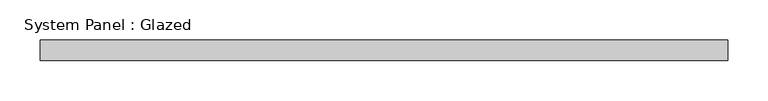
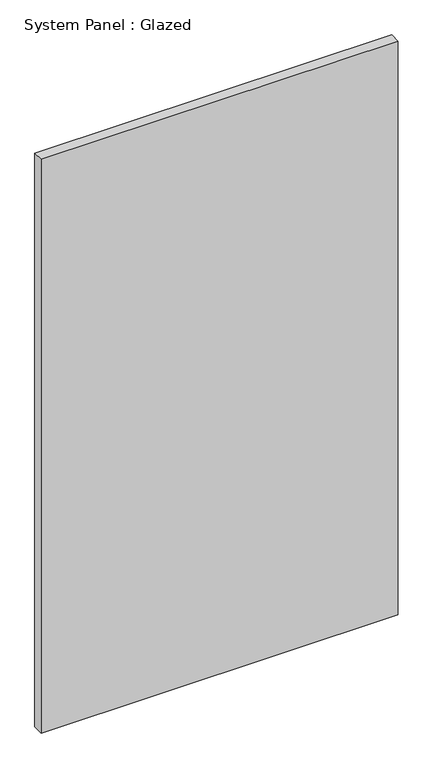
"""IFC4 building model written with IfcOpenShell, lengths in millimetres: plate geometry, System Panel : Glazed."""

from ifc_helpers import new_model, si_unit, origin, origin_with_axes, place, context, project, spatial, polyline, outline, extrude, source, transform, mapped, element, save


def system_panel_glazed_14014958(model_context):
    return source(origin(), model_context, "Body", "SweptSolid", [
        extrude(outline(polyline([(425.45, 19.05), (-425.45, 19.05), (-425.45, 44.45), (425.45, 44.45), (425.45, 19.05)])), origin_with_axes(), (0.0, 0.0, 1.0), 1444.0246189),
    ])


if __name__ == "__main__":
    model = new_model("IFC4")
    model_context = context("Model", 3, world=origin())
    ifc_project = project(units=[si_unit("LENGTHUNIT", "METRE", prefix="MILLI")], contexts=[model_context])
    site = spatial("IfcSite", under=ifc_project)
    building = spatial("IfcBuilding", under=site)
    placement = place(None, origin())
    system_panel_glazed_shape = system_panel_glazed_14014958(model_context)
    element("IfcPlate", 1, ObjectType="System Panel : Glazed", at=placement, inside=building, context=model_context, shape_type="MappedRepresentation", body=[
        mapped(system_panel_glazed_shape, transform((0.0, 0.0, 0.0), x_axis=(1.0, 0.0, 0.0), y_axis=(0.0, 1.0, 0.0), z_axis=(0.0, 0.0, 1.0))),
    ])
    save(model, "model.ifc")

# Revit data of these elements
# Type "System Panel : Glazed"
#   Construction Type Id = "GSP4R"
#   Analytic Construction = "1/8 in Pilkington single glazing"
#   Visual Light Transmittance = 0.9
#   Solar Heat Gain Coefficient = 0.86
#   Heat Transfer Coefficient (U) = 1.18115 BTU/(h·ft²·°F)
#   Define Thermal Properties by = 1
# Element 1 (IfcPlate, "System Panel : Glazed")
#   Materials on its faces: "Glass"
# Materials
#   "Glass": class "Glass", colour RGB 0 128 192, transparency 0.75, Description = "Soda Lime Glass", Cost = 0
